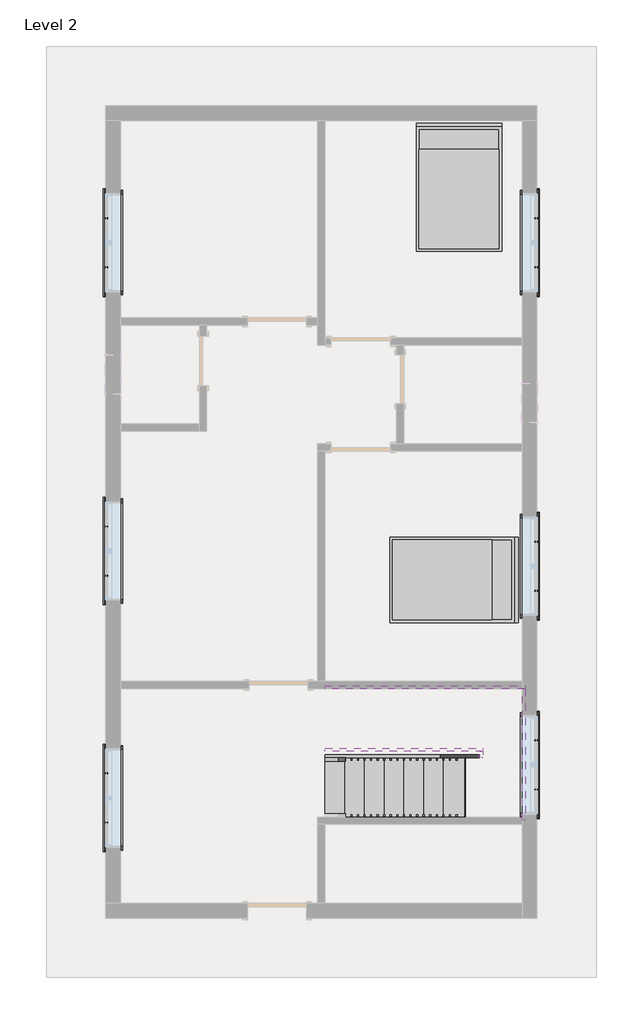
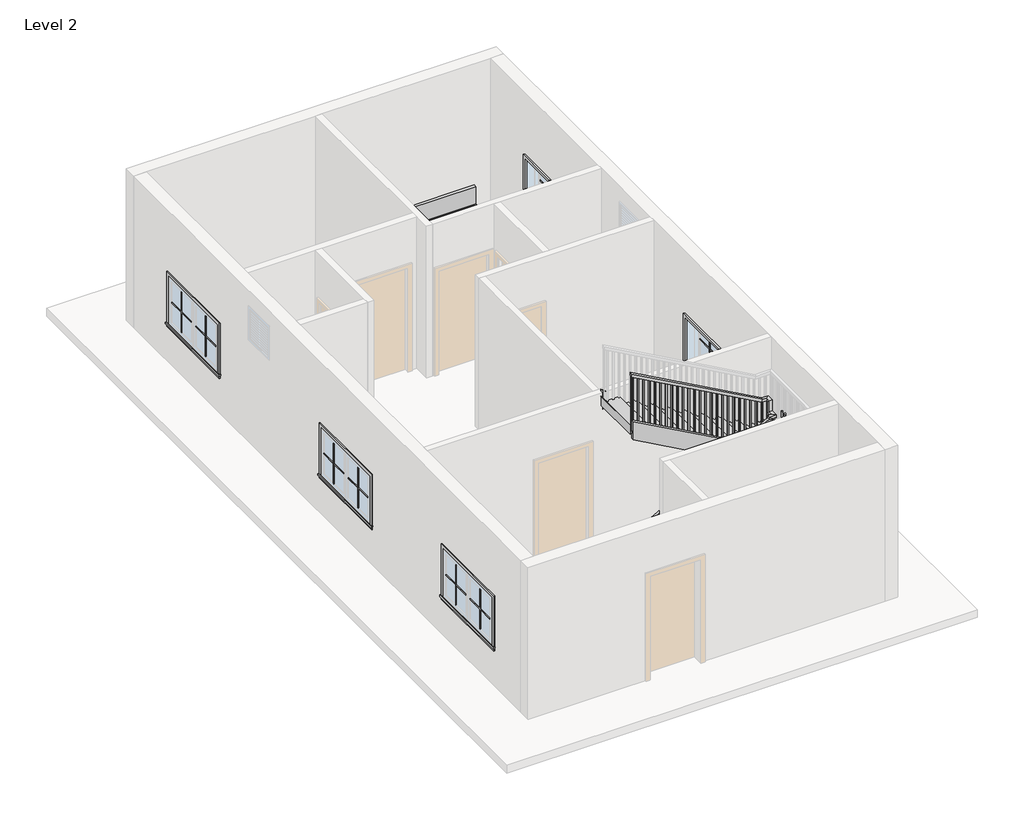
# One storey, part 3 of 3: 24 proxies, 6 members, 2 furniture elements, 1 railing, 1 stair flight.
"""IFC4 building model written with IfcOpenShell, lengths in millimetres."""

from ifc_helpers import new_model, si_unit, frame, origin, place, context, project, spatial, polyline, outline, extrude, faceted_brep, transform, mapped, element, save
from components import muntin_pattern_2x2_muntin_pattern_2x2_9352d081, muntin_pattern_2x2_muntin_pattern_2x2_5c2cbe28, trim_window_exterior_flat_with_sill_979bde60, trim_window_interior_flat_picture_frame_7883d11b, bed_17739_bed_17739_15c61121, stair_flight_21a7b5a9

model = new_model("IFC4")

# Units and contexts
model_context = context("Model", 3, world=origin())
ifc_project = project(units=[si_unit("LENGTHUNIT", "METRE", prefix="MILLI")], contexts=[model_context])

# Site, building, storey
site = spatial("IfcSite", under=ifc_project)
building = spatial("IfcBuilding", under=site)
storey = spatial("IfcBuildingStorey", under=building, Name="Level 2", Elevation=3048.0)

# Proxies
placement = place(None, origin())
muntin_pattern_2x2_muntin_pattern_2x2_shape = muntin_pattern_2x2_muntin_pattern_2x2_9352d081(model_context)
element("IfcBuildingElementProxy", 1, Name="Muntin Pattern_2x2 : Muntin Pattern_2x2", ObjectType="Muntin Pattern_2x2 : Muntin Pattern_2x2", at=placement, inside=storey, context=model_context, shape_type="MappedRepresentation", body=[
    mapped(muntin_pattern_2x2_muntin_pattern_2x2_shape, transform((-4579.34688, 3675.02881, 4032.25), x_axis=(0.0, 1.0, 0.0), y_axis=(-1.0, 0.0, 0.0), z_axis=(0.0, 0.0, 1.0))),
])
element("IfcBuildingElementProxy", 2, Name="Muntin Pattern_2x2 : Muntin Pattern_2x2", ObjectType="Muntin Pattern_2x2 : Muntin Pattern_2x2", at=placement, inside=storey, context=model_context, shape_type="MappedRepresentation", body=[
    mapped(muntin_pattern_2x2_muntin_pattern_2x2_shape, transform((-4579.34688, -1087.47119, 4032.25), x_axis=(0.0, 1.0, 0.0), y_axis=(-1.0, 0.0, 0.0), z_axis=(0.0, 0.0, 1.0))),
])
element("IfcBuildingElementProxy", 3, Name="Muntin Pattern_2x2 : Muntin Pattern_2x2", ObjectType="Muntin Pattern_2x2 : Muntin Pattern_2x2", at=placement, inside=storey, context=model_context, shape_type="MappedRepresentation", body=[
    mapped(muntin_pattern_2x2_muntin_pattern_2x2_shape, transform((-4579.34688, -4900.64619, 4032.25), x_axis=(0.0, 1.0, 0.0), y_axis=(-1.0, 0.0, 0.0), z_axis=(0.0, 0.0, 1.0))),
])
element("IfcBuildingElementProxy", 4, Name="Muntin Pattern_2x2 : Muntin Pattern_2x2", ObjectType="Muntin Pattern_2x2 : Muntin Pattern_2x2", at=placement, inside=storey, context=model_context, shape_type="MappedRepresentation", body=[
    mapped(muntin_pattern_2x2_muntin_pattern_2x2_shape, transform((2069.10312, -3630.64619, 4032.25), x_axis=(0.0, -1.0, 0.0), y_axis=(1.0, 0.0, 0.0), z_axis=(0.0, 0.0, 1.0))),
])
element("IfcBuildingElementProxy", 5, Name="Muntin Pattern_2x2 : Muntin Pattern_2x2", ObjectType="Muntin Pattern_2x2 : Muntin Pattern_2x2", at=placement, inside=storey, context=model_context, shape_type="MappedRepresentation", body=[
    mapped(muntin_pattern_2x2_muntin_pattern_2x2_shape, transform((2069.10312, 4433.85381, 4032.25), x_axis=(0.0, -1.0, 0.0), y_axis=(1.0, 0.0, 0.0), z_axis=(0.0, 0.0, 1.0))),
])
element("IfcBuildingElementProxy", 6, Name="Muntin Pattern_2x2 : Muntin Pattern_2x2", ObjectType="Muntin Pattern_2x2 : Muntin Pattern_2x2", at=placement, inside=storey, context=model_context, shape_type="MappedRepresentation", body=[
    mapped(muntin_pattern_2x2_muntin_pattern_2x2_shape, transform((2069.10312, -563.59619, 4032.25), x_axis=(0.0, -1.0, 0.0), y_axis=(1.0, 0.0, 0.0), z_axis=(0.0, 0.0, 1.0))),
])
muntin_pattern_2x2_muntin_pattern_2x2_2_shape = muntin_pattern_2x2_muntin_pattern_2x2_5c2cbe28(model_context)
element("IfcBuildingElementProxy", 7, Name="Muntin Pattern_2x2 : Muntin Pattern_2x2", ObjectType="Muntin Pattern_2x2 : Muntin Pattern_2x2", at=placement, inside=storey, context=model_context, shape_type="MappedRepresentation", body=[
    mapped(muntin_pattern_2x2_muntin_pattern_2x2_2_shape, transform((-4579.34688, 4433.85381, 4032.25), x_axis=(0.0, -1.0, 0.0), y_axis=(1.0, 0.0, 0.0), z_axis=(0.0, 0.0, 1.0))),
])
element("IfcBuildingElementProxy", 8, Name="Muntin Pattern_2x2 : Muntin Pattern_2x2", ObjectType="Muntin Pattern_2x2 : Muntin Pattern_2x2", at=placement, inside=storey, context=model_context, shape_type="MappedRepresentation", body=[
    mapped(muntin_pattern_2x2_muntin_pattern_2x2_2_shape, transform((-4579.34688, -328.64619, 4032.25), x_axis=(0.0, -1.0, 0.0), y_axis=(1.0, 0.0, 0.0), z_axis=(0.0, 0.0, 1.0))),
])
element("IfcBuildingElementProxy", 9, Name="Muntin Pattern_2x2 : Muntin Pattern_2x2", ObjectType="Muntin Pattern_2x2 : Muntin Pattern_2x2", at=placement, inside=storey, context=model_context, shape_type="MappedRepresentation", body=[
    mapped(muntin_pattern_2x2_muntin_pattern_2x2_2_shape, transform((-4579.34688, -4141.82119, 4032.25), x_axis=(0.0, -1.0, 0.0), y_axis=(1.0, 0.0, 0.0), z_axis=(0.0, 0.0, 1.0))),
])
element("IfcBuildingElementProxy", 10, Name="Muntin Pattern_2x2 : Muntin Pattern_2x2", ObjectType="Muntin Pattern_2x2 : Muntin Pattern_2x2", at=placement, inside=storey, context=model_context, shape_type="MappedRepresentation", body=[
    mapped(muntin_pattern_2x2_muntin_pattern_2x2_2_shape, transform((2069.10312, -4389.47119, 4032.25), x_axis=(0.0, 1.0, 0.0), y_axis=(-1.0, 0.0, 0.0), z_axis=(0.0, 0.0, 1.0))),
])
element("IfcBuildingElementProxy", 11, Name="Muntin Pattern_2x2 : Muntin Pattern_2x2", ObjectType="Muntin Pattern_2x2 : Muntin Pattern_2x2", at=placement, inside=storey, context=model_context, shape_type="MappedRepresentation", body=[
    mapped(muntin_pattern_2x2_muntin_pattern_2x2_2_shape, transform((2069.10312, 3675.02881, 4032.25), x_axis=(0.0, 1.0, 0.0), y_axis=(-1.0, 0.0, 0.0), z_axis=(0.0, 0.0, 1.0))),
])
element("IfcBuildingElementProxy", 12, Name="Muntin Pattern_2x2 : Muntin Pattern_2x2", ObjectType="Muntin Pattern_2x2 : Muntin Pattern_2x2", at=placement, inside=storey, context=model_context, shape_type="MappedRepresentation", body=[
    mapped(muntin_pattern_2x2_muntin_pattern_2x2_2_shape, transform((2069.10312, -1322.42119, 4032.25), x_axis=(0.0, 1.0, 0.0), y_axis=(-1.0, 0.0, 0.0), z_axis=(0.0, 0.0, 1.0))),
])
trim_window_exterior_flat_with_sill_shape = trim_window_exterior_flat_with_sill_979bde60(model_context)
element("IfcBuildingElementProxy", 13, Name="Trim-Window-Exterior-Flat : with Sill", ObjectType="Trim-Window-Exterior-Flat : with Sill", at=placement, inside=storey, context=model_context, shape_type="MappedRepresentation", body=[
    mapped(trim_window_exterior_flat_with_sill_shape, transform((-4588.87188, 4054.44131, 4876.8), x_axis=(0.0, -1.0, 0.0), y_axis=(0.0, 0.0, 1.0), z_axis=(-1.0, 0.0, 0.0))),
])
element("IfcBuildingElementProxy", 14, Name="Trim-Window-Exterior-Flat : with Sill", ObjectType="Trim-Window-Exterior-Flat : with Sill", at=placement, inside=storey, context=model_context, shape_type="MappedRepresentation", body=[
    mapped(trim_window_exterior_flat_with_sill_shape, transform((-4588.87188, -708.05869, 4876.8), x_axis=(0.0, -1.0, 0.0), y_axis=(0.0, 0.0, 1.0), z_axis=(-1.0, 0.0, 0.0))),
])
element("IfcBuildingElementProxy", 15, Name="Trim-Window-Exterior-Flat : with Sill", ObjectType="Trim-Window-Exterior-Flat : with Sill", at=placement, inside=storey, context=model_context, shape_type="MappedRepresentation", body=[
    mapped(trim_window_exterior_flat_with_sill_shape, transform((-4588.87188, -4521.23369, 4876.8), x_axis=(0.0, -1.0, 0.0), y_axis=(0.0, 0.0, 1.0), z_axis=(-1.0, 0.0, 0.0))),
])
element("IfcBuildingElementProxy", 16, Name="Trim-Window-Exterior-Flat : with Sill", ObjectType="Trim-Window-Exterior-Flat : with Sill", at=placement, inside=storey, context=model_context, shape_type="MappedRepresentation", body=[
    mapped(trim_window_exterior_flat_with_sill_shape, transform((2078.62812, -4010.05869, 4876.8), x_axis=(0.0, 1.0, 0.0), y_axis=(0.0, 0.0, 1.0), z_axis=(1.0, 0.0, 0.0))),
])
element("IfcBuildingElementProxy", 17, Name="Trim-Window-Exterior-Flat : with Sill", ObjectType="Trim-Window-Exterior-Flat : with Sill", at=placement, inside=storey, context=model_context, shape_type="MappedRepresentation", body=[
    mapped(trim_window_exterior_flat_with_sill_shape, transform((2078.62812, 4054.44131, 4876.8), x_axis=(0.0, 1.0, 0.0), y_axis=(0.0, 0.0, 1.0), z_axis=(1.0, 0.0, 0.0))),
])
element("IfcBuildingElementProxy", 18, Name="Trim-Window-Exterior-Flat : with Sill", ObjectType="Trim-Window-Exterior-Flat : with Sill", at=placement, inside=storey, context=model_context, shape_type="MappedRepresentation", body=[
    mapped(trim_window_exterior_flat_with_sill_shape, transform((2078.62812, -943.00869, 4876.8), x_axis=(0.0, 1.0, 0.0), y_axis=(0.0, 0.0, 1.0), z_axis=(1.0, 0.0, 0.0))),
])
trim_window_interior_flat_picture_frame_shape = trim_window_interior_flat_picture_frame_7883d11b(model_context)
element("IfcBuildingElementProxy", 19, Name="Trim-Window-Interior-Flat : Picture Frame", ObjectType="Trim-Window-Interior-Flat : Picture Frame", at=placement, inside=storey, context=model_context, shape_type="MappedRepresentation", body=[
    mapped(trim_window_interior_flat_picture_frame_shape, transform((-4360.27188, 4054.44131, 4876.8), x_axis=(0.0, 1.0, 0.0), y_axis=(0.0, 0.0, 1.0), z_axis=(1.0, 0.0, 0.0))),
])
element("IfcBuildingElementProxy", 20, Name="Trim-Window-Interior-Flat : Picture Frame", ObjectType="Trim-Window-Interior-Flat : Picture Frame", at=placement, inside=storey, context=model_context, shape_type="MappedRepresentation", body=[
    mapped(trim_window_interior_flat_picture_frame_shape, transform((-4360.27188, -708.05869, 4876.8), x_axis=(0.0, 1.0, 0.0), y_axis=(0.0, 0.0, 1.0), z_axis=(1.0, 0.0, 0.0))),
])
element("IfcBuildingElementProxy", 21, Name="Trim-Window-Interior-Flat : Picture Frame", ObjectType="Trim-Window-Interior-Flat : Picture Frame", at=placement, inside=storey, context=model_context, shape_type="MappedRepresentation", body=[
    mapped(trim_window_interior_flat_picture_frame_shape, transform((-4360.27188, -4521.23369, 4876.8), x_axis=(0.0, 1.0, 0.0), y_axis=(0.0, 0.0, 1.0), z_axis=(1.0, 0.0, 0.0))),
])
element("IfcBuildingElementProxy", 22, Name="Trim-Window-Interior-Flat : Picture Frame", ObjectType="Trim-Window-Interior-Flat : Picture Frame", at=placement, inside=storey, context=model_context, shape_type="MappedRepresentation", body=[
    mapped(trim_window_interior_flat_picture_frame_shape, transform((1850.02812, -4010.05869, 4876.8), x_axis=(0.0, -1.0, 0.0), y_axis=(0.0, 0.0, 1.0), z_axis=(-1.0, 0.0, 0.0))),
])
element("IfcBuildingElementProxy", 23, Name="Trim-Window-Interior-Flat : Picture Frame", ObjectType="Trim-Window-Interior-Flat : Picture Frame", at=placement, inside=storey, context=model_context, shape_type="MappedRepresentation", body=[
    mapped(trim_window_interior_flat_picture_frame_shape, transform((1850.02812, 4054.44131, 4876.8), x_axis=(0.0, -1.0, 0.0), y_axis=(0.0, 0.0, 1.0), z_axis=(-1.0, 0.0, 0.0))),
])
element("IfcBuildingElementProxy", 24, Name="Trim-Window-Interior-Flat : Picture Frame", ObjectType="Trim-Window-Interior-Flat : Picture Frame", at=placement, inside=storey, context=model_context, shape_type="MappedRepresentation", body=[
    mapped(trim_window_interior_flat_picture_frame_shape, transform((1850.02812, -943.00869, 4876.8), x_axis=(0.0, -1.0, 0.0), y_axis=(0.0, 0.0, 1.0), z_axis=(-1.0, 0.0, 0.0))),
])

# Furniture
bed_17739_bed_17739_shape = bed_17739_bed_17739_15c61121(model_context)
element("IfcFurniture", 25, ObjectType="Bed_17739 : Bed_17739", at=placement, inside=storey, context=model_context, shape_type="MappedRepresentation", body=[
    mapped(bed_17739_bed_17739_shape, transform((872.12812, 4886.29131, 3048.0), x_axis=(1.0, 0.0, 0.0), y_axis=(0.0, 1.0, 0.0), z_axis=(0.0, 0.0, 1.0))),
])
element("IfcFurniture", 26, ObjectType="Bed_17739 : Bed_17739", at=placement, inside=storey, context=model_context, shape_type="MappedRepresentation", body=[
    mapped(bed_17739_bed_17739_shape, transform((770.52812, -1152.55869, 3048.0), x_axis=(0.0, -1.0, 0.0), y_axis=(1.0, 0.0, 0.0), z_axis=(0.0, 0.0, 1.0))),
])

# Members
element("IfcMember", 27, ObjectType="Stringer - 2\" Width", at=placement, inside=storey, context=model_context, shape_type="SweptSolid", body=[
    extrude(outline(polyline([(3255.5983948, -1197.97188), (3048.0, -1197.97188), (3048.0, -944.0273772), (4233.3641651, 1189.62812), (4582.0428392, 1189.62812), (3255.5983948, -1197.97188)])), frame((0.0, -3902.10869, 0.0), z_axis=(0.0, 1.0, 0.0), x_axis=(0.0, 0.0, 1.0)), (0.0, 0.0, 1.0), 50.8),
])
element("IfcMember", 28, ObjectType="Stringer - 2\" Width", at=placement, inside=storey, context=model_context, shape_type="SweptSolid", body=[
    extrude(outline(polyline([(1240.42812, -3902.10869), (1189.62812, -3902.10869), (1189.62812, -3800.50869), (1240.42812, -3800.50869), (1240.42812, -3902.10869)])), frame((0.0, 0.0, 4343.4), z_axis=(0.0, 0.0, 1.0), x_axis=(1.0, 0.0, 0.0)), (0.0, 0.0, 1.0), 304.8),
])
element("IfcMember", 29, ObjectType="Stringer - 2\" Width", at=placement, inside=storey, context=model_context, shape_type="SweptSolid", body=[
    extrude(outline(polyline([(4430.9197207, 1240.42812), (4779.5983948, 1240.42812), (6134.2650614, -1197.97188), (5785.5863873, -1197.97188), (4430.9197207, 1240.42812)])), frame((0.0, -3800.50869, 0.0), z_axis=(0.0, 1.0, 0.0), x_axis=(0.0, 0.0, 1.0)), (0.0, 0.0, 1.0), 50.8),
])
element("IfcMember", 30, ObjectType="Stringer - 2\" Width", at=placement, inside=storey, context=model_context, shape_type="SweptSolid", body=[
    extrude(outline(polyline([(3255.5983948, -1197.97188), (3048.0, -1197.97188), (3048.0, -944.0273772), (4600.253054, 1850.02812), (4648.2, 1850.02812), (4648.2, 1308.7110094), (3255.5983948, -1197.97188)])), frame((0.0, -4867.30869, 0.0), z_axis=(0.0, 1.0, 0.0), x_axis=(0.0, 0.0, 1.0)), (0.0, 0.0, 1.0), 50.8),
])
element("IfcMember", 31, ObjectType="Stringer - 2\" Width", at=placement, inside=storey, context=model_context, shape_type="SweptSolid", body=[
    extrude(outline(polyline([(1900.82812, -4867.30869), (1850.02812, -4867.30869), (1850.02812, -2835.30869), (1900.82812, -2835.30869), (1900.82812, -4867.30869)])), frame((0.0, 0.0, 4343.4), z_axis=(0.0, 0.0, 1.0), x_axis=(1.0, 0.0, 0.0)), (0.0, 0.0, 1.0), 304.8),
])
element("IfcMember", 32, ObjectType="Stringer - 2\" Width", at=placement, inside=storey, context=model_context, shape_type="SweptSolid", body=[
    extrude(outline(polyline([(4343.4, 1900.82812), (4412.7095059, 1900.82812), (6134.2650614, -1197.97188), (5785.5863873, -1197.97188), (4343.4, 1397.9636172), (4343.4, 1900.82812)])), frame((0.0, -2835.30869, 0.0), z_axis=(0.0, 1.0, 0.0), x_axis=(0.0, 0.0, 1.0)), (0.0, 0.0, 1.0), 50.8),
])

# Railing
element("IfcRailing", 33, ObjectType="Handrail - Rectangular", at=placement, inside=storey, context=model_context, shape_type="SolidModel", body=[
    faceted_brep([(-1197.97188, -3902.10869, 4131.7333333), (-1197.97188, -3902.10869, 4073.620221), (-1197.97188, -3952.90869, 4073.620221), (-1197.97188, -3952.90869, 4131.7333333), (1164.22812, -3902.10869, 5444.0666667), (1215.02812, -3902.10869, 5414.1757765), (1215.02812, -3952.90869, 5414.1757765), (1164.22812, -3952.90869, 5444.0666667), (1164.22812, -3902.10869, 5486.4), (1215.02812, -3902.10869, 5435.6), (1215.02812, -3952.90869, 5435.6), (1164.22812, -3952.90869, 5486.4), (1240.42812, -3902.10869, 5486.4), (1240.42812, -3902.10869, 5435.6), (1291.22812, -3952.90869, 5435.6), (1291.22812, -3952.90869, 5486.4), (1240.42812, -3825.90869, 5486.4), (1240.42812, -3775.10869, 5435.6), (1291.22812, -3775.10869, 5435.6), (1291.22812, -3825.90869, 5486.4), (1240.42812, -3825.90869, 5698.0666667), (1240.42812, -3775.10869, 5647.2666667), (1291.22812, -3775.10869, 5647.2666667), (1291.22812, -3825.90869, 5698.0666667), (1240.42812, -3749.70869, 5698.0666667), (1240.42812, -3749.70869, 5647.2666667), (1291.22812, -3698.90869, 5647.2666667), (1291.22812, -3698.90869, 5698.0666667), (1164.22812, -3749.70869, 5698.0666667), (1151.0645177, -3749.70869, 5647.2666667), (1151.0645177, -3698.90869, 5647.2666667), (1164.22812, -3698.90869, 5698.0666667), (-1197.97188, -3749.70869, 7010.4), (-1197.97188, -3698.90869, 7010.4), (-1197.97188, -3698.90869, 6952.2868876), (-1197.97188, -3749.70869, 6952.2868876)], [[[0, 1, 2, 3]], [[1, 0, 4, 5]], [[2, 1, 5, 6]], [[3, 2, 6, 7]], [[0, 3, 7, 4]], [[5, 4, 8, 9]], [[6, 5, 9, 10]], [[7, 6, 10, 11]], [[4, 7, 11, 8]], [[9, 8, 12, 13]], [[10, 9, 13, 14]], [[11, 10, 14, 15]], [[8, 11, 15, 12]], [[13, 12, 16, 17]], [[14, 13, 17, 18]], [[15, 14, 18, 19]], [[12, 15, 19, 16]], [[17, 16, 20, 21]], [[18, 17, 21, 22]], [[19, 18, 22, 23]], [[16, 19, 23, 20]], [[21, 20, 24, 25]], [[22, 21, 25, 26]], [[23, 22, 26, 27]], [[20, 23, 27, 24]], [[25, 24, 28, 29]], [[26, 25, 29, 30]], [[27, 26, 30, 31]], [[24, 27, 31, 28]], [[32, 33, 34, 35]], [[29, 28, 32, 35]], [[30, 29, 35, 34]], [[31, 30, 34, 33]], [[28, 31, 33, 32]]]),
    extrude(outline(polyline([(6943.4674432, -1182.09688), (5926.6666667, -1182.09688), (5926.6666667, -1163.04688), (6932.8841099, -1163.04688), (6943.4674432, -1182.09688)])), frame((0.0, -3733.83369, 0.0), z_axis=(0.0, 1.0, 0.0), x_axis=(0.0, 0.0, 1.0)), (0.0, 0.0, 1.0), 19.05),
    extrude(outline(polyline([(6887.0229988, -1080.49688), (5926.6666667, -1080.49688), (5926.6666667, -1061.44688), (6876.4396654, -1061.44688), (6887.0229988, -1080.49688)])), frame((0.0, -3733.83369, 0.0), z_axis=(0.0, 1.0, 0.0), x_axis=(0.0, 0.0, 1.0)), (0.0, 0.0, 1.0), 19.05),
    extrude(outline(polyline([(6830.5785543, -978.89688), (5926.6666667, -978.89688), (5926.6666667, -959.84688), (6819.995221, -959.84688), (6830.5785543, -978.89688)])), frame((0.0, -3733.83369, 0.0), z_axis=(0.0, 1.0, 0.0), x_axis=(0.0, 0.0, 1.0)), (0.0, 0.0, 1.0), 19.05),
    extrude(outline(polyline([(6774.1341099, -877.29688), (5757.3333333, -877.29688), (5757.3333333, -858.24688), (6763.5507765, -858.24688), (6774.1341099, -877.29688)])), frame((0.0, -3733.83369, 0.0), z_axis=(0.0, 1.0, 0.0), x_axis=(0.0, 0.0, 1.0)), (0.0, 0.0, 1.0), 19.05),
    extrude(outline(polyline([(6717.6896654, -775.69688), (5757.3333333, -775.69688), (5757.3333333, -756.64688), (6707.1063321, -756.64688), (6717.6896654, -775.69688)])), frame((0.0, -3733.83369, 0.0), z_axis=(0.0, 1.0, 0.0), x_axis=(0.0, 0.0, 1.0)), (0.0, 0.0, 1.0), 19.05),
    extrude(outline(polyline([(6661.245221, -674.09688), (5757.3333333, -674.09688), (5757.3333333, -655.04688), (6650.6618876, -655.04688), (6661.245221, -674.09688)])), frame((0.0, -3733.83369, 0.0), z_axis=(0.0, 1.0, 0.0), x_axis=(0.0, 0.0, 1.0)), (0.0, 0.0, 1.0), 19.05),
    extrude(outline(polyline([(6604.8007765, -572.49688), (5588.0, -572.49688), (5588.0, -553.44688), (6594.2174432, -553.44688), (6604.8007765, -572.49688)])), frame((0.0, -3733.83369, 0.0), z_axis=(0.0, 1.0, 0.0), x_axis=(0.0, 0.0, 1.0)), (0.0, 0.0, 1.0), 19.05),
    extrude(outline(polyline([(6548.3563321, -470.89688), (5588.0, -470.89688), (5588.0, -451.84688), (6537.7729988, -451.84688), (6548.3563321, -470.89688)])), frame((0.0, -3733.83369, 0.0), z_axis=(0.0, 1.0, 0.0), x_axis=(0.0, 0.0, 1.0)), (0.0, 0.0, 1.0), 19.05),
    extrude(outline(polyline([(6491.9118876, -369.29688), (5588.0, -369.29688), (5588.0, -350.24688), (6481.3285543, -350.24688), (6491.9118876, -369.29688)])), frame((0.0, -3733.83369, 0.0), z_axis=(0.0, 1.0, 0.0), x_axis=(0.0, 0.0, 1.0)), (0.0, 0.0, 1.0), 19.05),
    extrude(outline(polyline([(6435.4674432, -267.69688), (5418.6666667, -267.69688), (5418.6666667, -248.64688), (6424.8841099, -248.64688), (6435.4674432, -267.69688)])), frame((0.0, -3733.83369, 0.0), z_axis=(0.0, 1.0, 0.0), x_axis=(0.0, 0.0, 1.0)), (0.0, 0.0, 1.0), 19.05),
    extrude(outline(polyline([(6379.0229988, -166.09688), (5418.6666667, -166.09688), (5418.6666667, -147.04688), (6368.4396654, -147.04688), (6379.0229988, -166.09688)])), frame((0.0, -3733.83369, 0.0), z_axis=(0.0, 1.0, 0.0), x_axis=(0.0, 0.0, 1.0)), (0.0, 0.0, 1.0), 19.05),
    extrude(outline(polyline([(6322.5785543, -64.49688), (5418.6666667, -64.49688), (5418.6666667, -45.44688), (6311.995221, -45.44688), (6322.5785543, -64.49688)])), frame((0.0, -3733.83369, 0.0), z_axis=(0.0, 1.0, 0.0), x_axis=(0.0, 0.0, 1.0)), (0.0, 0.0, 1.0), 19.05),
    extrude(outline(polyline([(6266.1341099, 37.10312), (5249.3333333, 37.10312), (5249.3333333, 56.15312), (6255.5507765, 56.15312), (6266.1341099, 37.10312)])), frame((0.0, -3733.83369, 0.0), z_axis=(0.0, 1.0, 0.0), x_axis=(0.0, 0.0, 1.0)), (0.0, 0.0, 1.0), 19.05),
    extrude(outline(polyline([(6209.6896654, 138.70312), (5249.3333333, 138.70312), (5249.3333333, 157.75312), (6199.1063321, 157.75312), (6209.6896654, 138.70312)])), frame((0.0, -3733.83369, 0.0), z_axis=(0.0, 1.0, 0.0), x_axis=(0.0, 0.0, 1.0)), (0.0, 0.0, 1.0), 19.05),
    extrude(outline(polyline([(6153.245221, 240.30312), (5249.3333333, 240.30312), (5249.3333333, 259.35312), (6142.6618876, 259.35312), (6153.245221, 240.30312)])), frame((0.0, -3733.83369, 0.0), z_axis=(0.0, 1.0, 0.0), x_axis=(0.0, 0.0, 1.0)), (0.0, 0.0, 1.0), 19.05),
    extrude(outline(polyline([(6096.8007765, 341.90312), (5080.0, 341.90312), (5080.0, 360.95312), (6086.2174432, 360.95312), (6096.8007765, 341.90312)])), frame((0.0, -3733.83369, 0.0), z_axis=(0.0, 1.0, 0.0), x_axis=(0.0, 0.0, 1.0)), (0.0, 0.0, 1.0), 19.05),
    extrude(outline(polyline([(6040.3563321, 443.50312), (5080.0, 443.50312), (5080.0, 462.55312), (6029.7729988, 462.55312), (6040.3563321, 443.50312)])), frame((0.0, -3733.83369, 0.0), z_axis=(0.0, 1.0, 0.0), x_axis=(0.0, 0.0, 1.0)), (0.0, 0.0, 1.0), 19.05),
    extrude(outline(polyline([(5983.9118876, 545.10312), (5080.0, 545.10312), (5080.0, 564.15312), (5973.3285543, 564.15312), (5983.9118876, 545.10312)])), frame((0.0, -3733.83369, 0.0), z_axis=(0.0, 1.0, 0.0), x_axis=(0.0, 0.0, 1.0)), (0.0, 0.0, 1.0), 19.05),
    extrude(outline(polyline([(5927.4674432, 646.70312), (4910.6666667, 646.70312), (4910.6666667, 665.75312), (5916.8841099, 665.75312), (5927.4674432, 646.70312)])), frame((0.0, -3733.83369, 0.0), z_axis=(0.0, 1.0, 0.0), x_axis=(0.0, 0.0, 1.0)), (0.0, 0.0, 1.0), 19.05),
    extrude(outline(polyline([(5871.0229988, 748.30312), (4910.6666667, 748.30312), (4910.6666667, 767.35312), (5860.4396654, 767.35312), (5871.0229988, 748.30312)])), frame((0.0, -3733.83369, 0.0), z_axis=(0.0, 1.0, 0.0), x_axis=(0.0, 0.0, 1.0)), (0.0, 0.0, 1.0), 19.05),
    extrude(outline(polyline([(5814.5785543, 849.90312), (4910.6666667, 849.90312), (4910.6666667, 868.95312), (5803.995221, 868.95312), (5814.5785543, 849.90312)])), frame((0.0, -3733.83369, 0.0), z_axis=(0.0, 1.0, 0.0), x_axis=(0.0, 0.0, 1.0)), (0.0, 0.0, 1.0), 19.05),
    extrude(outline(polyline([(5758.1341099, 951.50312), (4741.3333333, 951.50312), (4741.3333333, 970.55312), (5747.5507765, 970.55312), (5758.1341099, 951.50312)])), frame((0.0, -3733.83369, 0.0), z_axis=(0.0, 1.0, 0.0), x_axis=(0.0, 0.0, 1.0)), (0.0, 0.0, 1.0), 19.05),
    extrude(outline(polyline([(5701.6896654, 1053.10312), (4741.3333333, 1053.10312), (4741.3333333, 1072.15312), (5691.1063321, 1072.15312), (5701.6896654, 1053.10312)])), frame((0.0, -3733.83369, 0.0), z_axis=(0.0, 1.0, 0.0), x_axis=(0.0, 0.0, 1.0)), (0.0, 0.0, 1.0), 19.05),
    extrude(outline(polyline([(5645.245221, 1154.70312), (4741.3333333, 1154.70312), (4741.3333333, 1173.75312), (5634.6618876, 1173.75312), (5645.245221, 1154.70312)])), frame((0.0, -3733.83369, 0.0), z_axis=(0.0, 1.0, 0.0), x_axis=(0.0, 0.0, 1.0)), (0.0, 0.0, 1.0), 19.05),
    extrude(outline(polyline([(1256.30312, -3835.43369), (1256.30312, -3816.38369), (1275.35312, -3816.38369), (1275.35312, -3835.43369), (1256.30312, -3835.43369)])), frame((0.0, 0.0, 4572.0), z_axis=(0.0, 0.0, 1.0), x_axis=(1.0, 0.0, 0.0)), (0.0, 0.0, 1.0), 863.6),
    extrude(outline(polyline([(1230.90312, -3917.98369), (1249.95312, -3917.98369), (1249.95312, -3937.03369), (1230.90312, -3937.03369), (1230.90312, -3917.98369)])), frame((0.0, 0.0, 4572.0), z_axis=(0.0, 0.0, 1.0), x_axis=(1.0, 0.0, 0.0)), (0.0, 0.0, 1.0), 863.6),
    extrude(outline(polyline([(5366.5507765, 1129.30312), (4402.6666667, 1129.30312), (4402.6666667, 1148.35312), (5377.1341099, 1148.35312), (5366.5507765, 1129.30312)])), frame((0.0, -3937.03369, 0.0), z_axis=(0.0, 1.0, 0.0), x_axis=(0.0, 0.0, 1.0)), (0.0, 0.0, 1.0), 19.05),
    extrude(outline(polyline([(5310.1063321, 1027.70312), (4402.6666667, 1027.70312), (4402.6666667, 1046.75312), (5320.6896654, 1046.75312), (5310.1063321, 1027.70312)])), frame((0.0, -3937.03369, 0.0), z_axis=(0.0, 1.0, 0.0), x_axis=(0.0, 0.0, 1.0)), (0.0, 0.0, 1.0), 19.05),
    extrude(outline(polyline([(5253.6618876, 926.10312), (4402.6666667, 926.10312), (4402.6666667, 945.15312), (5264.245221, 945.15312), (5253.6618876, 926.10312)])), frame((0.0, -3937.03369, 0.0), z_axis=(0.0, 1.0, 0.0), x_axis=(0.0, 0.0, 1.0)), (0.0, 0.0, 1.0), 19.05),
    extrude(outline(polyline([(5197.2174432, 824.50312), (4233.3333333, 824.50312), (4233.3333333, 843.55312), (5207.8007765, 843.55312), (5197.2174432, 824.50312)])), frame((0.0, -3937.03369, 0.0), z_axis=(0.0, 1.0, 0.0), x_axis=(0.0, 0.0, 1.0)), (0.0, 0.0, 1.0), 19.05),
    extrude(outline(polyline([(5140.7729988, 722.90312), (4233.3333333, 722.90312), (4233.3333333, 741.95312), (5151.3563321, 741.95312), (5140.7729988, 722.90312)])), frame((0.0, -3937.03369, 0.0), z_axis=(0.0, 1.0, 0.0), x_axis=(0.0, 0.0, 1.0)), (0.0, 0.0, 1.0), 19.05),
    extrude(outline(polyline([(5084.3285543, 621.30312), (4233.3333333, 621.30312), (4233.3333333, 640.35312), (5094.9118876, 640.35312), (5084.3285543, 621.30312)])), frame((0.0, -3937.03369, 0.0), z_axis=(0.0, 1.0, 0.0), x_axis=(0.0, 0.0, 1.0)), (0.0, 0.0, 1.0), 19.05),
    extrude(outline(polyline([(5027.8841099, 519.70312), (4064.0, 519.70312), (4064.0, 538.75312), (5038.4674432, 538.75312), (5027.8841099, 519.70312)])), frame((0.0, -3937.03369, 0.0), z_axis=(0.0, 1.0, 0.0), x_axis=(0.0, 0.0, 1.0)), (0.0, 0.0, 1.0), 19.05),
    extrude(outline(polyline([(4971.4396654, 418.10312), (4064.0, 418.10312), (4064.0, 437.15312), (4982.0229988, 437.15312), (4971.4396654, 418.10312)])), frame((0.0, -3937.03369, 0.0), z_axis=(0.0, 1.0, 0.0), x_axis=(0.0, 0.0, 1.0)), (0.0, 0.0, 1.0), 19.05),
    extrude(outline(polyline([(4914.995221, 316.50312), (4064.0, 316.50312), (4064.0, 335.55312), (4925.5785543, 335.55312), (4914.995221, 316.50312)])), frame((0.0, -3937.03369, 0.0), z_axis=(0.0, 1.0, 0.0), x_axis=(0.0, 0.0, 1.0)), (0.0, 0.0, 1.0), 19.05),
    extrude(outline(polyline([(4858.5507765, 214.90312), (3894.6666667, 214.90312), (3894.6666667, 233.95312), (4869.1341099, 233.95312), (4858.5507765, 214.90312)])), frame((0.0, -3937.03369, 0.0), z_axis=(0.0, 1.0, 0.0), x_axis=(0.0, 0.0, 1.0)), (0.0, 0.0, 1.0), 19.05),
    extrude(outline(polyline([(4802.1063321, 113.30312), (3894.6666667, 113.30312), (3894.6666667, 132.35312), (4812.6896654, 132.35312), (4802.1063321, 113.30312)])), frame((0.0, -3937.03369, 0.0), z_axis=(0.0, 1.0, 0.0), x_axis=(0.0, 0.0, 1.0)), (0.0, 0.0, 1.0), 19.05),
    extrude(outline(polyline([(4745.6618876, 11.70312), (3894.6666667, 11.70312), (3894.6666667, 30.75312), (4756.245221, 30.75312), (4745.6618876, 11.70312)])), frame((0.0, -3937.03369, 0.0), z_axis=(0.0, 1.0, 0.0), x_axis=(0.0, 0.0, 1.0)), (0.0, 0.0, 1.0), 19.05),
    extrude(outline(polyline([(4689.2174432, -89.89688), (3725.3333333, -89.89688), (3725.3333333, -70.84688), (4699.8007765, -70.84688), (4689.2174432, -89.89688)])), frame((0.0, -3937.03369, 0.0), z_axis=(0.0, 1.0, 0.0), x_axis=(0.0, 0.0, 1.0)), (0.0, 0.0, 1.0), 19.05),
    extrude(outline(polyline([(4632.7729988, -191.49688), (3725.3333333, -191.49688), (3725.3333333, -172.44688), (4643.3563321, -172.44688), (4632.7729988, -191.49688)])), frame((0.0, -3937.03369, 0.0), z_axis=(0.0, 1.0, 0.0), x_axis=(0.0, 0.0, 1.0)), (0.0, 0.0, 1.0), 19.05),
    extrude(outline(polyline([(4576.3285543, -293.09688), (3725.3333333, -293.09688), (3725.3333333, -274.04688), (4586.9118876, -274.04688), (4576.3285543, -293.09688)])), frame((0.0, -3937.03369, 0.0), z_axis=(0.0, 1.0, 0.0), x_axis=(0.0, 0.0, 1.0)), (0.0, 0.0, 1.0), 19.05),
    extrude(outline(polyline([(4519.8841099, -394.69688), (3556.0, -394.69688), (3556.0, -375.64688), (4530.4674432, -375.64688), (4519.8841099, -394.69688)])), frame((0.0, -3937.03369, 0.0), z_axis=(0.0, 1.0, 0.0), x_axis=(0.0, 0.0, 1.0)), (0.0, 0.0, 1.0), 19.05),
    extrude(outline(polyline([(4463.4396654, -496.29688), (3556.0, -496.29688), (3556.0, -477.24688), (4474.0229988, -477.24688), (4463.4396654, -496.29688)])), frame((0.0, -3937.03369, 0.0), z_axis=(0.0, 1.0, 0.0), x_axis=(0.0, 0.0, 1.0)), (0.0, 0.0, 1.0), 19.05),
    extrude(outline(polyline([(4406.995221, -597.89688), (3556.0, -597.89688), (3556.0, -578.84688), (4417.5785543, -578.84688), (4406.995221, -597.89688)])), frame((0.0, -3937.03369, 0.0), z_axis=(0.0, 1.0, 0.0), x_axis=(0.0, 0.0, 1.0)), (0.0, 0.0, 1.0), 19.05),
    extrude(outline(polyline([(4350.5507765, -699.49688), (3386.6666667, -699.49688), (3386.6666667, -680.44688), (4361.1341099, -680.44688), (4350.5507765, -699.49688)])), frame((0.0, -3937.03369, 0.0), z_axis=(0.0, 1.0, 0.0), x_axis=(0.0, 0.0, 1.0)), (0.0, 0.0, 1.0), 19.05),
    extrude(outline(polyline([(4294.1063321, -801.09688), (3386.6666667, -801.09688), (3386.6666667, -782.04688), (4304.6896654, -782.04688), (4294.1063321, -801.09688)])), frame((0.0, -3937.03369, 0.0), z_axis=(0.0, 1.0, 0.0), x_axis=(0.0, 0.0, 1.0)), (0.0, 0.0, 1.0), 19.05),
    extrude(outline(polyline([(4237.6618876, -902.69688), (3386.6666667, -902.69688), (3386.6666667, -883.64688), (4248.245221, -883.64688), (4237.6618876, -902.69688)])), frame((0.0, -3937.03369, 0.0), z_axis=(0.0, 1.0, 0.0), x_axis=(0.0, 0.0, 1.0)), (0.0, 0.0, 1.0), 19.05),
    extrude(outline(polyline([(4181.2174432, -1004.29688), (3217.3333333, -1004.29688), (3217.3333333, -985.24688), (4191.8007765, -985.24688), (4181.2174432, -1004.29688)])), frame((0.0, -3937.03369, 0.0), z_axis=(0.0, 1.0, 0.0), x_axis=(0.0, 0.0, 1.0)), (0.0, 0.0, 1.0), 19.05),
    extrude(outline(polyline([(4124.7729988, -1105.89688), (3217.3333333, -1105.89688), (3217.3333333, -1086.84688), (4135.3563321, -1086.84688), (4124.7729988, -1105.89688)])), frame((0.0, -3937.03369, 0.0), z_axis=(0.0, 1.0, 0.0), x_axis=(0.0, 0.0, 1.0)), (0.0, 0.0, 1.0), 19.05),
    extrude(outline(polyline([(1256.30312, -3733.83369), (1256.30312, -3714.78369), (1275.35312, -3714.78369), (1275.35312, -3733.83369), (1256.30312, -3733.83369)])), frame((0.0, 0.0, 4572.0), z_axis=(0.0, 0.0, 1.0), x_axis=(1.0, 0.0, 0.0)), (0.0, 0.0, 1.0), 1075.2666667),
    extrude(outline(polyline([(1256.30312, -3917.98369), (1275.35312, -3917.98369), (1275.35312, -3937.03369), (1256.30312, -3937.03369), (1256.30312, -3917.98369)])), frame((0.0, 0.0, 4572.0), z_axis=(0.0, 0.0, 1.0), x_axis=(1.0, 0.0, 0.0)), (0.0, 0.0, 1.0), 863.6),
    extrude(outline(polyline([(6952.2868876, -1197.97188), (5926.6666667, -1197.97188), (5926.6666667, -1178.92188), (6941.7035543, -1178.92188), (6952.2868876, -1197.97188)])), frame((0.0, -3733.83369, 0.0), z_axis=(0.0, 1.0, 0.0), x_axis=(0.0, 0.0, 1.0)), (0.0, 0.0, 1.0), 19.05),
    extrude(outline(polyline([(4073.620221, -1197.97188), (3217.3333333, -1197.97188), (3217.3333333, -1178.92188), (4084.2035543, -1178.92188), (4073.620221, -1197.97188)])), frame((0.0, -3937.03369, 0.0), z_axis=(0.0, 1.0, 0.0), x_axis=(0.0, 0.0, 1.0)), (0.0, 0.0, 1.0), 19.05),
])

# Stair flight
stair_flight_shape = stair_flight_21a7b5a9(model_context)
element("IfcStairFlight", 34, ObjectType="2\" Tread 1\" Nosing 1/4\" Riser", at=placement, inside=storey, context=model_context, shape_type="MappedRepresentation", body=[
    mapped(stair_flight_shape, transform((0.0, 0.0, 0.0), x_axis=(1.0, 0.0, 0.0), y_axis=(0.0, 1.0, 0.0), z_axis=(0.0, 0.0, 1.0))),
])

save(model, "model.ifc")

# Revit data of these elements
# Type "Muntin Pattern_2x2 : Muntin Pattern_2x2"
#   Width [instance default] = 4' - 0"
#   Thickness = 0' - 0 1/2"
#   Height [instance default] = 4' - 0"
#   Distance = 0' - 0 3/4"
#   Interior Material [instance default] = none
#   Exterior Material [instance default] = none
#   Default Elevation = 0
# Type "Trim-Window-Exterior-Flat : with Sill"
#   Trim Width = 0' - 2 1/4"
#   Trim Thickness_Picture Frame = 0' - 1 1/4"
#   Trim Thickness_with Sill = 0' - 0 3/4"
#   Sill Thickness = 0' - 1 1/4"
#   Opening Width [instance default] = 2' - 0"
#   Opening Height [instance default] = 3' - 0"
#   Default Elevation = 4' - 0"
#   Sill = yes
#   Picture Frame = no
#   Trim Material [instance default] = none
# Type "Trim-Window-Interior-Flat : Picture Frame"
#   Trim Thickness_Picture Frame = 0' - 1 1/4"
#   Trim Width = 0' - 2 1/4"
#   Trim Thickness_with Sill = 0' - 0 3/4"
#   Sill Thickness = 0' - 1 1/4"
#   Opening Width [instance default] = 2' - 0"
#   Opening Height [instance default] = 3' - 0"
#   Default Elevation = 4' - 0"
#   Sill = no
#   Picture Frame = yes
#   Trim Material [instance default] = none
# Type "Bed_17739 : Bed_17739"
#   Default Elevation = 0
# Type "Handrail - Rectangular"
#   Assembly Code = "C2010400"
#   built-in parameter 1008612 = 0.0416667 (stored number, unit not read)
#   built-in parameter 1008611 = 0.0416667 (stored number, unit not read)
#   built-in parameter 1008609 = 0.333333 (stored number, unit not read)
#   built-in parameter 1008604 = 0.166667 (stored number, unit not read)
#   built-in parameter 1008603 = 0.166667 (stored number, unit not read)
#   Railing Height = 3' - 0"
#   built-in parameter 1008630 = 2
#   built-in parameter 1008610 = 2
#   built-in parameter 1008618 = Baluster - Square : 3/4"
# Elements 1, 2, 3, 4, 5, 6, 7, 8, 9, 10, 11, 12 (IfcBuildingElementProxy, "Muntin Pattern_2x2 : Muntin Pattern_2x2")
#   Width = 2' - 0 5/8"
#   Height = 2' - 6 1/2"
#   Interior Material = Wood - Stained
#   Exterior Material = Clad - White
#   Phase Created = New Construction
#   Materials on its faces: "Clad - White", "Wood - Stained"
# Elements 13, 14, 15, 16, 17, 18 (IfcBuildingElementProxy, "Trim-Window-Exterior-Flat : with Sill")
#   Opening Width = 5' - 0"
#   Opening Height = 3' - 0"
#   Trim Material = Clad - White
#   Phase Created = New Construction
#   Materials on its faces: "Clad - White"
# Elements 19, 20, 21, 22, 23, 24 (IfcBuildingElementProxy, "Trim-Window-Interior-Flat : Picture Frame")
#   Opening Width = 5' - 0"
#   Opening Height = 3' - 0"
#   Trim Material = Wood - Stained
#   Phase Created = New Construction
#   Materials on its faces: "Wood - Stained"
# Elements 25, 26 (IfcFurniture, "Bed_17739 : Bed_17739")
#   Phase Created = New Construction
#   Materials on its faces: "legs", "sheets", "bed frame", "Blanket"
# Elements 27, 28, 29, 30, 31, 32 (IfcMember, "Stringer - 2\" Width")
#   Phase Created = New Construction
# Element 33 (IfcRailing, "Handrail - Rectangular")
#   Phase Created = New Construction
# Element 34 (IfcStairFlight, "2\" Tread 1\" Nosing 1/4\" Riser")
#   Phase Created = New Construction
# Materials
#   "Clad - White": class "Wood", colour RGB 242 242 238, transparency 0, Cost = 0
#   "Wood - Stained": class "Wood", colour RGB 224 178 126, transparency 0, Cost = 0
#   "legs": colour RGB 90 73 37, transparency 0, Cost = 0
#   "sheets": colour RGB 200 195 176, transparency 0, Cost = 0
#   "bed frame": colour RGB 90 73 37, transparency 0, Cost = 0
#   "Blanket": class "System", colour RGB 59 0 1, transparency 0, Cost = 0
